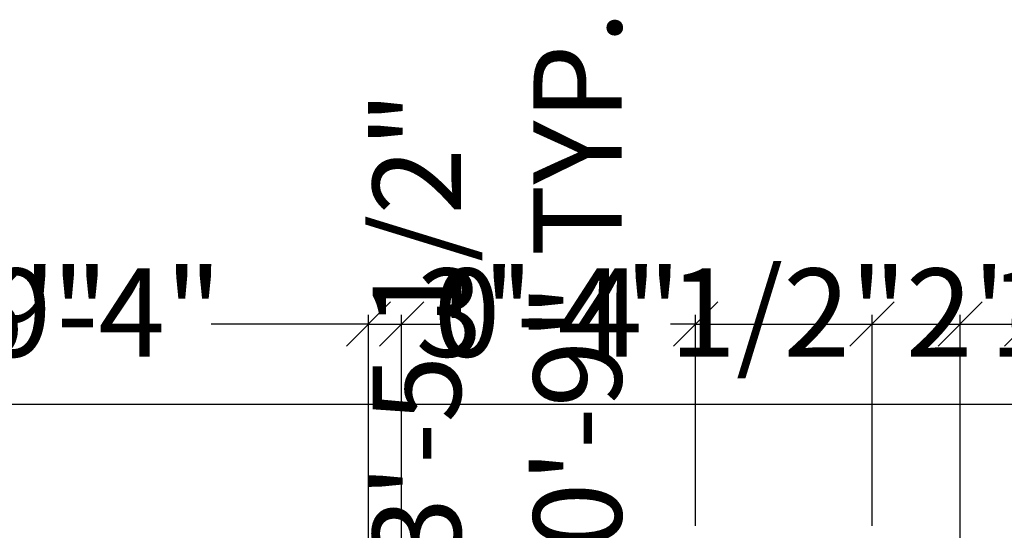
# Model space of a CAD drawing. Units: inches. Extents: x 2371 to 3019, y 129 to 700.
# Tile 7 of 14: x 2445 to 2579, y 631 to 700. Entities that reach past the tile are written whole.
import ezdxf

# ---------------------------------------------------------------- set-up
doc = ezdxf.new("R2010")
doc.units = ezdxf.units.IN
doc.layers.add('A-ANNO-DIMS', color=2, linetype='Continuous', lineweight=18)
doc.styles.get("Standard").update_dxf_attribs({"font": 'arial.ttf'})
doc.dimstyles.new('ISO-25', dxfattribs={"dimtxt": 12, "dimasz": 6, "dimexe": 1.25, "dimexo": 0.625, "dimtad": 0, "dimdec": 1, "dimlunit": 3, "dimtxsty": 'Standard', "dimblk": 'OBLIQUE', "dimblk1": 'ORIGIN2', "dimblk2": 'OBLIQUE', "dimcen": 2.5, "dimadec": 0, "dimazin": 0, "dimtfac": 1, "dimtdec": 1, "dimtmove": 0, "dimatfit": 3, "dimldrblk": 'OBLIQUE', "dimfxl": 1, "dimarcsym": 0})

# ---------------------------------------------------------------- blocks, each defined once
blk = doc.blocks.new('_Oblique')
at = {"color": 0, "linetype": 'ByBlock', "lineweight": -2}
blk.add_line((-0.5, -0.5), (0.5, 0.5), dxfattribs=at)
blk = doc.blocks.new('*D14')
at = {"layer": 'A-ANNO-DIMS', "color": 0, "lineweight": -2, "transparency": 16777216}
for p, q in [((2407.11, 631.6), (2407.11, 649.37)), ((2923.11, 631.6), (2923.11, 649.37)), ((2407.11, 648.12), (2643.63, 648.12)), ((2923.11, 648.12), (2686.58, 648.12))]:
    blk.add_line(p, q, dxfattribs=at)
at = {"layer": 'Defpoints', "color": 0, "lineweight": 25, "transparency": 16777216}
for p in [(2923.11, 648.12), (2407.11, 630.98), (2923.11, 630.98)]:
    blk.add_point(p, dxfattribs=at)
at = {"layer": 'A-ANNO-DIMS', "color": 0, "lineweight": -2, "transparency": 16777216, "xscale": 6, "yscale": 6, "zscale": 6, "rotation": 180}
blk.add_blockref('_Oblique', (2407.11, 648.12), dxfattribs=at)
at = {"layer": 'A-ANNO-DIMS', "color": 0, "lineweight": -2, "transparency": 16777216, "xscale": 6, "yscale": 6, "zscale": 6}
blk.add_blockref('_Oblique', (2923.11, 648.12), dxfattribs=at)
at = {"layer": 'A-ANNO-DIMS', "color": 0, "transparency": 16777216, "insert": (2665.11, 648.12), "char_height": 12, "width": 20.8486, "attachment_point": 5}
blk.add_mtext('43\'-0"', dxfattribs=at)
blk = doc.blocks.new('_Origin2')
at = {"color": 0, "linetype": 'ByBlock', "lineweight": -2}
blk.add_line((-0.5, 0), (-1, 0), dxfattribs=at)
for radius in [0.5, 0.25]:
    blk.add_circle((0, 0), radius, dxfattribs=at)
blk = doc.blocks.new('*D30')
at = {"layer": 'A-ANNO-DIMS', "color": 0, "lineweight": -2, "transparency": 16777216}
for p, q in [((2505.18, 612.41), (2505.18, 609.58)), ((2519.88, 612.41), (2519.88, 609.58)), ((2505.18, 610.83), (2519.88, 610.83)), ((2519.88, 610.83), (2525.88, 610.83))]:
    blk.add_line(p, q, dxfattribs=at)
at = {"layer": 'Defpoints', "color": 0, "lineweight": 25, "transparency": 16777216}
for p in [(2505.18, 613.03), (2519.88, 613.03), (2519.88, 610.83)]:
    blk.add_point(p, dxfattribs=at)
at = {"layer": 'A-ANNO-DIMS', "color": 0, "lineweight": -2, "transparency": 16777216, "xscale": 6, "yscale": 6, "zscale": 6, "rotation": 180}
blk.add_blockref('_Oblique', (2505.18, 610.83), dxfattribs=at)
at = {"layer": 'A-ANNO-DIMS', "color": 0, "lineweight": -2, "transparency": 16777216, "xscale": 6, "yscale": 6, "zscale": 6}
blk.add_blockref('_Oblique', (2519.88, 610.83), dxfattribs=at)
at = {"layer": 'A-ANNO-DIMS', "color": 0, "transparency": 16777216, "insert": (2645.95, 610.83), "char_height": 12, "attachment_point": 5}
blk.add_mtext('SHOWER MIXER 1\'-2 1/2" TYP.', dxfattribs=at)
blk = doc.blocks.new('*D31')
at = {"layer": 'A-ANNO-DIMS', "color": 0, "lineweight": -2, "transparency": 16777216}
for p, q in [((2522.09, 621.8), (2522.09, 627.8)), ((2520.51, 621.8), (2523.34, 621.8)), ((2522.09, 613.03), (2522.09, 621.8)), ((2520.51, 613.03), (2523.34, 613.03))]:
    blk.add_line(p, q, dxfattribs=at)
at = {"layer": 'Defpoints', "color": 0, "lineweight": 25, "transparency": 16777216}
for p in [(2519.88, 621.8), (2522.09, 621.8), (2519.88, 613.03)]:
    blk.add_point(p, dxfattribs=at)
at = {"layer": 'A-ANNO-DIMS', "color": 0, "lineweight": -2, "transparency": 16777216, "xscale": 6, "yscale": 6, "zscale": 6}
for p, rotation in [((2522.09, 621.8), 90), ((2522.09, 613.03), 270)]:
    blk.add_blockref('_Oblique', p, dxfattribs=dict(at, rotation=rotation))
at = {"layer": 'A-ANNO-DIMS', "color": 0, "transparency": 16777216, "insert": (2522.09, 665), "char_height": 12, "attachment_point": 5, "rotation": 90}
blk.add_mtext('0\'-9" TYP.', dxfattribs=at)
blk = doc.blocks.new('*D34')
at = {"layer": 'A-ANNO-DIMS', "color": 0, "lineweight": -2, "transparency": 16777216}
for p, q in [((2407.11, 631.6), (2407.11, 660.28)), ((2416.11, 622.6), (2416.11, 660.28)), ((2407.11, 659.03), (2416.11, 659.03)), ((2416.11, 659.03), (2422.11, 659.03))]:
    blk.add_line(p, q, dxfattribs=at)
at = {"layer": 'Defpoints', "color": 0, "lineweight": 25, "transparency": 16777216}
for p in [(2416.11, 659.03), (2407.11, 630.98), (2416.11, 621.98)]:
    blk.add_point(p, dxfattribs=at)
at = {"layer": 'A-ANNO-DIMS', "color": 0, "lineweight": -2, "transparency": 16777216, "xscale": 6, "yscale": 6, "zscale": 6, "rotation": 180}
blk.add_blockref('_Oblique', (2407.11, 659.03), dxfattribs=at)
at = {"layer": 'A-ANNO-DIMS', "color": 0, "lineweight": -2, "transparency": 16777216, "xscale": 6, "yscale": 6, "zscale": 6}
blk.add_blockref('_Oblique', (2416.11, 659.03), dxfattribs=at)
at = {"layer": 'A-ANNO-DIMS', "color": 0, "transparency": 16777216, "insert": (2438.68, 659.03), "char_height": 12, "attachment_point": 5}
blk.add_mtext('0\'-9"', dxfattribs=at)
blk = doc.blocks.new('*D35')
at = {"layer": 'A-ANNO-DIMS', "color": 0, "lineweight": -2, "transparency": 16777216}
for p, q in [((2416.11, 622.6), (2416.11, 660.28)), ((2492.11, 622.6), (2492.11, 660.28)), ((2416.11, 659.03), (2437.5, 659.03)), ((2492.11, 659.03), (2470.71, 659.03))]:
    blk.add_line(p, q, dxfattribs=at)
at = {"layer": 'Defpoints', "color": 0, "lineweight": 25, "transparency": 16777216}
for p in [(2492.11, 659.03), (2416.11, 621.98), (2492.11, 621.98)]:
    blk.add_point(p, dxfattribs=at)
at = {"layer": 'A-ANNO-DIMS', "color": 0, "lineweight": -2, "transparency": 16777216, "xscale": 6, "yscale": 6, "zscale": 6, "rotation": 180}
blk.add_blockref('_Oblique', (2416.11, 659.03), dxfattribs=at)
at = {"layer": 'A-ANNO-DIMS', "color": 0, "lineweight": -2, "transparency": 16777216, "xscale": 6, "yscale": 6, "zscale": 6}
blk.add_blockref('_Oblique', (2492.11, 659.03), dxfattribs=at)
at = {"layer": 'A-ANNO-DIMS', "color": 0, "transparency": 16777216, "insert": (2454.11, 659.03), "char_height": 12, "attachment_point": 5}
blk.add_mtext('6\'-4"', dxfattribs=at)
blk = doc.blocks.new('*D36')
at = {"layer": 'A-ANNO-DIMS', "color": 0, "lineweight": -2, "transparency": 16777216}
for p, q in [((2492.11, 622.6), (2492.11, 660.28)), ((2496.61, 622.6), (2496.61, 660.28)), ((2492.11, 659.03), (2496.61, 659.03)), ((2496.61, 659.03), (2502.61, 659.03))]:
    blk.add_line(p, q, dxfattribs=at)
at = {"layer": 'Defpoints', "color": 0, "lineweight": 25, "transparency": 16777216}
for p in [(2496.61, 659.03), (2492.11, 621.98), (2496.61, 621.98)]:
    blk.add_point(p, dxfattribs=at)
at = {"layer": 'A-ANNO-DIMS', "color": 0, "lineweight": -2, "transparency": 16777216, "xscale": 6, "yscale": 6, "zscale": 6, "rotation": 180}
blk.add_blockref('_Oblique', (2492.11, 659.03), dxfattribs=at)
at = {"layer": 'A-ANNO-DIMS', "color": 0, "lineweight": -2, "transparency": 16777216, "xscale": 6, "yscale": 6, "zscale": 6}
blk.add_blockref('_Oblique', (2496.61, 659.03), dxfattribs=at)
at = {"layer": 'A-ANNO-DIMS', "color": 0, "transparency": 16777216, "insert": (2533.16, 659.03), "char_height": 12, "attachment_point": 5}
blk.add_mtext('0\'-4 1/2"', dxfattribs=at)
blk = doc.blocks.new('*D37')
at = {"layer": 'A-ANNO-DIMS', "color": 0, "lineweight": -2, "transparency": 16777216}
for p, q in [((2496.61, 622.6), (2496.61, 660.28)), ((2536.61, 631.6), (2536.61, 660.28)), ((2496.61, 659.03), (2500.03, 659.03)), ((2536.61, 659.03), (2533.18, 659.03))]:
    blk.add_line(p, q, dxfattribs=at)
at = {"layer": 'Defpoints', "color": 0, "lineweight": 25, "transparency": 16777216}
for p in [(2536.61, 659.03), (2536.61, 630.98), (2496.61, 621.98)]:
    blk.add_point(p, dxfattribs=at)
at = {"layer": 'A-ANNO-DIMS', "color": 0, "lineweight": -2, "transparency": 16777216, "xscale": 6, "yscale": 6, "zscale": 6, "rotation": 180}
blk.add_blockref('_Oblique', (2496.61, 659.03), dxfattribs=at)
at = {"layer": 'A-ANNO-DIMS', "color": 0, "lineweight": -2, "transparency": 16777216, "xscale": 6, "yscale": 6, "zscale": 6}
blk.add_blockref('_Oblique', (2536.61, 659.03), dxfattribs=at)
at = {"layer": 'A-ANNO-DIMS', "color": 0, "transparency": 16777216, "insert": (2516.61, 659.03), "char_height": 12, "attachment_point": 5}
blk.add_mtext('3\'-4"', dxfattribs=at)
blk = doc.blocks.new('*D38')
at = {"layer": 'A-ANNO-DIMS', "color": 0, "lineweight": -2, "transparency": 16777216}
for p, q in [((2536.61, 631.6), (2536.61, 660.28)), ((2560.61, 631.6), (2560.61, 660.28)), ((2536.61, 659.03), (2560.61, 659.03)), ((2560.61, 659.03), (2566.61, 659.03))]:
    blk.add_line(p, q, dxfattribs=at)
at = {"layer": 'Defpoints', "color": 0, "lineweight": 25, "transparency": 16777216}
for p in [(2560.61, 659.03), (2536.61, 630.98), (2560.61, 630.98)]:
    blk.add_point(p, dxfattribs=at)
at = {"layer": 'A-ANNO-DIMS', "color": 0, "lineweight": -2, "transparency": 16777216, "xscale": 6, "yscale": 6, "zscale": 6, "rotation": 180}
blk.add_blockref('_Oblique', (2536.61, 659.03), dxfattribs=at)
at = {"layer": 'A-ANNO-DIMS', "color": 0, "lineweight": -2, "transparency": 16777216, "xscale": 6, "yscale": 6, "zscale": 6}
blk.add_blockref('_Oblique', (2560.61, 659.03), dxfattribs=at)
at = {"layer": 'A-ANNO-DIMS', "color": 0, "transparency": 16777216, "insert": (2583.28, 659.03), "char_height": 12, "attachment_point": 5}
blk.add_mtext('2\'-0"', dxfattribs=at)
blk = doc.blocks.new('*D39')
at = {"layer": 'A-ANNO-DIMS', "color": 0, "lineweight": -2, "transparency": 16777216}
for p, q in [((2560.61, 631.6), (2560.61, 660.28)), ((2572.61, 622.6), (2572.61, 660.28)), ((2560.61, 659.03), (2572.61, 659.03)), ((2572.61, 659.03), (2578.61, 659.03))]:
    blk.add_line(p, q, dxfattribs=at)
at = {"layer": 'Defpoints', "color": 0, "lineweight": 25, "transparency": 16777216}
for p in [(2572.61, 659.03), (2560.61, 630.98), (2572.61, 621.98)]:
    blk.add_point(p, dxfattribs=at)
at = {"layer": 'A-ANNO-DIMS', "color": 0, "lineweight": -2, "transparency": 16777216, "xscale": 6, "yscale": 6, "zscale": 6, "rotation": 180}
blk.add_blockref('_Oblique', (2560.61, 659.03), dxfattribs=at)
at = {"layer": 'A-ANNO-DIMS', "color": 0, "lineweight": -2, "transparency": 16777216, "xscale": 6, "yscale": 6, "zscale": 6}
blk.add_blockref('_Oblique', (2572.61, 659.03), dxfattribs=at)
at = {"layer": 'A-ANNO-DIMS', "color": 0, "transparency": 16777216, "insert": (2594.61, 659.03), "char_height": 12, "attachment_point": 5}
blk.add_mtext('1\'-0"', dxfattribs=at)
blk = doc.blocks.new('*D40')
at = {"layer": 'A-ANNO-DIMS', "color": 0, "lineweight": -2, "transparency": 16777216}
for p, q in [((2572.61, 622.6), (2572.61, 660.28)), ((2581.61, 622.6), (2581.61, 660.28)), ((2572.61, 659.03), (2581.61, 659.03)), ((2581.61, 659.03), (2587.61, 659.03))]:
    blk.add_line(p, q, dxfattribs=at)
at = {"layer": 'Defpoints', "color": 0, "lineweight": 25, "transparency": 16777216}
for p in [(2581.61, 659.03), (2572.61, 621.98), (2581.61, 621.98)]:
    blk.add_point(p, dxfattribs=at)
at = {"layer": 'A-ANNO-DIMS', "color": 0, "lineweight": -2, "transparency": 16777216, "xscale": 6, "yscale": 6, "zscale": 6, "rotation": 180}
blk.add_blockref('_Oblique', (2572.61, 659.03), dxfattribs=at)
at = {"layer": 'A-ANNO-DIMS', "color": 0, "lineweight": -2, "transparency": 16777216, "xscale": 6, "yscale": 6, "zscale": 6}
blk.add_blockref('_Oblique', (2581.61, 659.03), dxfattribs=at)
at = {"layer": 'A-ANNO-DIMS', "color": 0, "transparency": 16777216, "insert": (2604.18, 659.03), "char_height": 12, "attachment_point": 5}
blk.add_mtext('0\'-9"', dxfattribs=at)
blk = doc.blocks.new('*D78')
at = {"layer": 'A-ANNO-DIMS', "color": 0, "lineweight": -2, "transparency": 16777216}
for p, q in [((2500.23, 621.98), (2500.23, 627.98)), ((2527.66, 621.98), (2498.98, 621.98)), ((2500.23, 580.36), (2500.23, 621.98)), ((2527.66, 580.36), (2498.98, 580.36))]:
    blk.add_line(p, q, dxfattribs=at)
at = {"layer": 'Defpoints', "color": 0, "lineweight": 25, "transparency": 16777216}
for p in [(2500.23, 621.98), (2528.28, 621.98), (2528.28, 580.36)]:
    blk.add_point(p, dxfattribs=at)
at = {"layer": 'A-ANNO-DIMS', "color": 0, "lineweight": -2, "transparency": 16777216, "xscale": 6, "yscale": 6, "zscale": 6}
for p, rotation in [((2500.23, 621.98), 90), ((2500.23, 580.36), 270)]:
    blk.add_blockref('_Oblique', p, dxfattribs=dict(at, rotation=rotation))
at = {"layer": 'A-ANNO-DIMS', "color": 0, "transparency": 16777216, "insert": (2500.23, 658.53), "char_height": 12, "attachment_point": 5, "rotation": 90}
blk.add_mtext('3\'-5 1/2"', dxfattribs=at)

msp = doc.modelspace()

# ---------------------------------------------------------------- dimensions: what is measured, and where the dimension line sits
at = {"layer": 'A-ANNO-DIMS'}
dim = msp.add_linear_dim(base=(2522.09, 621.8), p1=(2519.88, 613.03), p2=(2519.88, 621.8), angle=90, text='<> TYP.', dimstyle='ISO-25', override={"dimdec": 1, "dimrnd": 0, "dimzin": 1, "dimlunit": 4, "dimfrac": 2}, dxfattribs=at)
dim.commit()
dim.dimension.update_dxf_attribs({"geometry": '*D31', "text_midpoint": (2522.09, 665)})
dim = msp.add_linear_dim(base=(2500.23, 621.98), p1=(2528.28, 580.36), p2=(2528.28, 621.98), angle=90, dimstyle='ISO-25', override={"dimdec": 1, "dimlfac": 1, "dimrnd": 0, "dimzin": 1, "dimdsep": 46, "dimlunit": 4, "dimfrac": 2}, dxfattribs=at)
dim.commit()
dim.dimension.update_dxf_attribs({"geometry": '*D78', "text_midpoint": (2500.23, 658.53)})
for base, p1, p2, picture, middle in [((2496.61, 659.03), (2492.11, 621.98), (2496.61, 621.98), '*D36', (2533.16, 659.03)), ((2416.11, 659.03), (2407.11, 630.98), (2416.11, 621.98), '*D34', (2438.68, 659.03)), ((2492.11, 659.03), (2416.11, 621.98), (2492.11, 621.98), '*D35', (2454.11, 659.03)), ((2536.61, 659.03), (2496.61, 621.98), (2536.61, 630.98), '*D37', (2516.61, 659.03)), ((2560.61, 659.03), (2536.61, 630.98), (2560.61, 630.98), '*D38', (2583.28, 659.03)), ((2572.61, 659.03), (2560.61, 630.98), (2572.61, 621.98), '*D39', (2594.61, 659.03)), ((2581.61, 659.03), (2572.61, 621.98), (2581.61, 621.98), '*D40', (2604.18, 659.03))]:
    dim = msp.add_linear_dim(base=base, p1=p1, p2=p2, dimstyle='ISO-25', override={"dimdec": 1, "dimlfac": 1, "dimrnd": 0, "dimzin": 1, "dimdsep": 46, "dimlunit": 4, "dimfrac": 2}, dxfattribs=at)
    dim.commit()
    dim.dimension.update_dxf_attribs({"geometry": picture, "text_midpoint": middle})
for base, p1, p2, text, override, picture, middle in [((2519.88, 610.83), (2505.18, 613.03), (2519.88, 613.03), 'SHOWER MIXER <> TYP.', {"dimdec": 1, "dimrnd": 0, "dimzin": 1, "dimlunit": 4, "dimfrac": 2}, '*D30', (2645.95, 610.83)), ((2923.11, 648.12), (2407.11, 630.98), (2923.11, 630.98), '43\'-0"', {"dimclrd": 0, "dimclre": 0, "dimclrt": 0}, '*D14', (2665.11, 648.12))]:
    dim = msp.add_linear_dim(base=base, p1=p1, p2=p2, text=text, dimstyle='ISO-25', override=override, dxfattribs=at)
    dim.commit()
    dim.dimension.update_dxf_attribs({"geometry": picture, "text_midpoint": middle})

doc.saveas('drawing.dxf')
